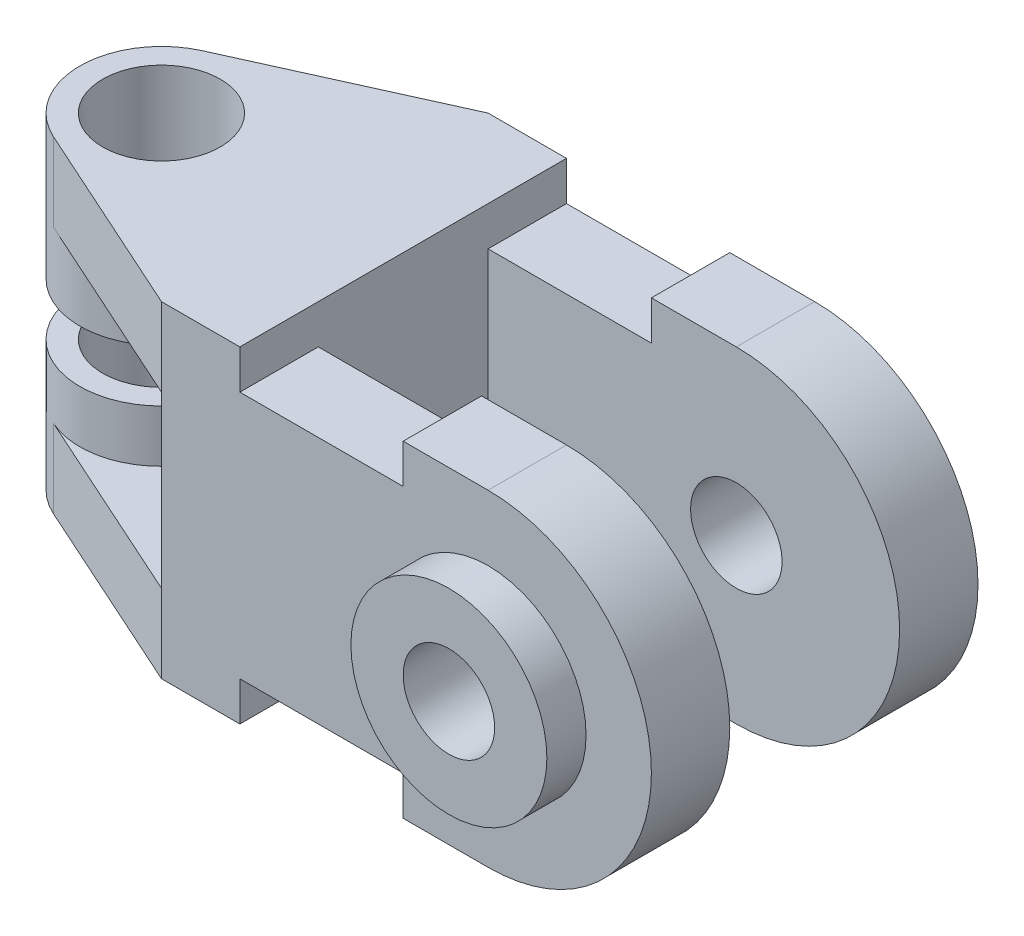
ISO-10303-21;
HEADER;
FILE_DESCRIPTION(('STEP AP214'),'2;1');
FILE_NAME('part.step','',(''),(''),'','','');
FILE_SCHEMA(('AUTOMOTIVE_DESIGN { 1 0 10303 214 1 1 1 1 }'));
ENDSEC;
DATA;
#1=APPLICATION_CONTEXT('core data for automotive mechanical design processes');
#2=APPLICATION_PROTOCOL_DEFINITION('international standard','automotive_design',2000,#1);
#3=PRODUCT_CONTEXT('',#1,'mechanical');
#4=PRODUCT('Part','Part','',(#3));
#5=PRODUCT_RELATED_PRODUCT_CATEGORY('part','',(#4));
#6=PRODUCT_DEFINITION_FORMATION('','',#4);
#7=PRODUCT_DEFINITION_CONTEXT('part definition',#1,'design');
#8=PRODUCT_DEFINITION('design','',#6,#7);
#9=PRODUCT_DEFINITION_SHAPE('','',#8);
#10=(LENGTH_UNIT() NAMED_UNIT(*) SI_UNIT(.MILLI.,.METRE.));
#11=(NAMED_UNIT(*) PLANE_ANGLE_UNIT() SI_UNIT($,.RADIAN.));
#12=(NAMED_UNIT(*) SI_UNIT($,.STERADIAN.) SOLID_ANGLE_UNIT());
#13=UNCERTAINTY_MEASURE_WITH_UNIT(LENGTH_MEASURE(1.E-05),#10,'distance_accuracy_value','');
#14=(GEOMETRIC_REPRESENTATION_CONTEXT(3) GLOBAL_UNCERTAINTY_ASSIGNED_CONTEXT((#13)) GLOBAL_UNIT_ASSIGNED_CONTEXT((#10,
#11,#12)) REPRESENTATION_CONTEXT('',''));
#15=CARTESIAN_POINT('',(0.,0.,0.));
#16=DIRECTION('',(0.,0.,1.));
#17=DIRECTION('',(1.,0.,0.));
#18=AXIS2_PLACEMENT_3D('',#15,#16,#17);
#19=CARTESIAN_POINT('',(0.,0.,12.));
#20=DIRECTION('',(1.,0.,0.));
#21=DIRECTION('',(0.,0.,-1.));
#22=AXIS2_PLACEMENT_3D('',#19,#20,#21);
#23=PLANE('',#22);
#24=DIRECTION('',(0.,0.,-1.));
#25=VECTOR('',#24,1.);
#26=CARTESIAN_POINT('',(0.,12.,0.));
#27=LINE('',#26,#25);
#28=CARTESIAN_POINT('',(0.,12.,12.));
#29=VERTEX_POINT('',#28);
#30=CARTESIAN_POINT('',(0.,12.,-38.));
#31=VERTEX_POINT('',#30);
#32=EDGE_CURVE('E62',#29,#31,#27,.T.);
#33=ORIENTED_EDGE('',*,*,#32,.F.);
#34=DIRECTION('',(0.,-1.,0.));
#35=VECTOR('',#34,1.);
#36=CARTESIAN_POINT('',(0.,0.,12.));
#37=LINE('',#36,#35);
#38=CARTESIAN_POINT('',(0.,38.,12.));
#39=VERTEX_POINT('',#38);
#40=EDGE_CURVE('E411',#39,#29,#37,.T.);
#41=ORIENTED_EDGE('',*,*,#40,.F.);
#42=DIRECTION('',(0.,0.,-1.));
#43=VECTOR('',#42,1.);
#44=CARTESIAN_POINT('',(0.,38.,-38.));
#45=LINE('',#44,#43);
#46=CARTESIAN_POINT('',(0.,38.,-38.));
#47=VERTEX_POINT('',#46);
#48=EDGE_CURVE('E265',#39,#47,#45,.T.);
#49=ORIENTED_EDGE('',*,*,#48,.T.);
#50=DIRECTION('',(0.,-1.,0.));
#51=VECTOR('',#50,1.);
#52=CARTESIAN_POINT('',(0.,50.,-38.));
#53=LINE('',#52,#51);
#54=EDGE_CURVE('E354',#47,#31,#53,.T.);
#55=ORIENTED_EDGE('',*,*,#54,.T.);
#56=EDGE_LOOP('',(#33,#41,#49,#55));
#57=FACE_BOUND('',#56,.T.);
#58=ADVANCED_FACE('F50',(#57),#23,.F.);
#59=CARTESIAN_POINT('',(12.,0.,12.));
#60=DIRECTION('',(0.,1.,0.));
#61=DIRECTION('',(0.,0.,1.));
#62=AXIS2_PLACEMENT_3D('',#59,#60,#61);
#63=PLANE('',#62);
#64=CARTESIAN_POINT('',(-24.9999999999965,0.,-13.));
#65=DIRECTION('',(0.,-1.,0.));
#66=DIRECTION('',(0.,0.,-1.));
#67=AXIS2_PLACEMENT_3D('',#64,#65,#66);
#68=CIRCLE('',#67,8.99999999999664);
#69=CARTESIAN_POINT('',(-24.9999999999965,0.,-21.9999999999966));
#70=VERTEX_POINT('',#69);
#71=EDGE_CURVE('E479',#70,#70,#68,.T.);
#72=ORIENTED_EDGE('',*,*,#71,.F.);
#73=EDGE_LOOP('',(#72));
#74=FACE_BOUND('',#73,.T.);
#75=DIRECTION('',(1.,0.,0.));
#76=VECTOR('',#75,1.);
#77=CARTESIAN_POINT('',(12.,0.,12.));
#78=LINE('',#77,#76);
#79=CARTESIAN_POINT('',(0.,0.,12.));
#80=VERTEX_POINT('',#79);
#81=CARTESIAN_POINT('',(12.,0.,12.));
#82=VERTEX_POINT('',#81);
#83=EDGE_CURVE('E249',#80,#82,#78,.T.);
#84=ORIENTED_EDGE('',*,*,#83,.F.);
#85=DIRECTION('',(-0.911437827766088,0.,-0.41143782776628));
#86=VECTOR('',#85,1.);
#87=CARTESIAN_POINT('',(-4.50000000000115,0.,9.96862696659558));
#88=LINE('',#87,#86);
#89=CARTESIAN_POINT('',(-30.1429728470736,0.,-1.60702715292695));
#90=VERTEX_POINT('',#89);
#91=EDGE_CURVE('E241',#80,#90,#88,.T.);
#92=ORIENTED_EDGE('',*,*,#91,.T.);
#93=CARTESIAN_POINT('',(-24.9999999999965,0.,-13.));
#94=DIRECTION('',(0.,-1.,0.));
#95=DIRECTION('',(0.,0.,-1.));
#96=AXIS2_PLACEMENT_3D('',#93,#94,#95);
#97=CIRCLE('',#96,12.4999999999966);
#98=CARTESIAN_POINT('',(-30.1429728470734,0.,-24.3929728470703));
#99=VERTEX_POINT('',#98);
#100=EDGE_CURVE('E224',#90,#99,#97,.T.);
#101=ORIENTED_EDGE('',*,*,#100,.T.);
#102=DIRECTION('',(-0.911437827766056,0.,0.41143782776635));
#103=VECTOR('',#102,1.);
#104=CARTESIAN_POINT('',(-14.2500000000056,0.,-31.5673187275505));
#105=LINE('',#104,#103);
#106=CARTESIAN_POINT('',(0.,0.,-38.));
#107=VERTEX_POINT('',#106);
#108=EDGE_CURVE('E255',#107,#99,#105,.T.);
#109=ORIENTED_EDGE('',*,*,#108,.F.);
#110=DIRECTION('',(-1.,0.,0.));
#111=VECTOR('',#110,1.);
#112=CARTESIAN_POINT('',(12.,0.,-38.));
#113=LINE('',#112,#111);
#114=CARTESIAN_POINT('',(12.,0.,-38.));
#115=VERTEX_POINT('',#114);
#116=EDGE_CURVE('E380',#115,#107,#113,.T.);
#117=ORIENTED_EDGE('',*,*,#116,.F.);
#118=DIRECTION('',(0.,0.,-1.));
#119=VECTOR('',#118,1.);
#120=CARTESIAN_POINT('',(12.,0.,12.));
#121=LINE('',#120,#119);
#122=EDGE_CURVE('E368',#82,#115,#121,.T.);
#123=ORIENTED_EDGE('',*,*,#122,.F.);
#124=EDGE_LOOP('',(#84,#92,#101,#109,#117,#123));
#125=FACE_BOUND('',#124,.T.);
#126=ADVANCED_FACE('F47',(#74,#125),#63,.F.);
#127=CARTESIAN_POINT('',(37.,6.,12.));
#128=DIRECTION('',(0.,1.,0.));
#129=DIRECTION('',(0.,0.,1.));
#130=AXIS2_PLACEMENT_3D('',#127,#128,#129);
#131=PLANE('',#130);
#132=DIRECTION('',(1.,0.,0.));
#133=VECTOR('',#132,1.);
#134=CARTESIAN_POINT('',(37.,6.,0.));
#135=LINE('',#134,#133);
#136=CARTESIAN_POINT('',(12.,6.,0.));
#137=VERTEX_POINT('',#136);
#138=CARTESIAN_POINT('',(37.,6.,0.));
#139=VERTEX_POINT('',#138);
#140=EDGE_CURVE('E383',#137,#139,#135,.T.);
#141=ORIENTED_EDGE('',*,*,#140,.T.);
#142=DIRECTION('',(0.,0.,-1.));
#143=VECTOR('',#142,1.);
#144=CARTESIAN_POINT('',(37.,6.,12.));
#145=LINE('',#144,#143);
#146=CARTESIAN_POINT('',(37.,6.,12.));
#147=VERTEX_POINT('',#146);
#148=EDGE_CURVE('E449',#147,#139,#145,.T.);
#149=ORIENTED_EDGE('',*,*,#148,.F.);
#150=DIRECTION('',(1.,0.,0.));
#151=VECTOR('',#150,1.);
#152=CARTESIAN_POINT('',(37.,6.,12.));
#153=LINE('',#152,#151);
#154=CARTESIAN_POINT('',(12.,6.,12.));
#155=VERTEX_POINT('',#154);
#156=EDGE_CURVE('E392',#155,#147,#153,.T.);
#157=ORIENTED_EDGE('',*,*,#156,.F.);
#158=DIRECTION('',(0.,0.,-1.));
#159=VECTOR('',#158,1.);
#160=CARTESIAN_POINT('',(12.,6.,12.));
#161=LINE('',#160,#159);
#162=EDGE_CURVE('E453',#155,#137,#161,.T.);
#163=ORIENTED_EDGE('',*,*,#162,.T.);
#164=EDGE_LOOP('',(#141,#149,#157,#163));
#165=FACE_BOUND('',#164,.T.);
#166=ADVANCED_FACE('F505',(#165),#131,.F.);
#167=CARTESIAN_POINT('',(37.,0.,12.));
#168=DIRECTION('',(1.,0.,0.));
#169=DIRECTION('',(0.,0.,-1.));
#170=AXIS2_PLACEMENT_3D('',#167,#168,#169);
#171=PLANE('',#170);
#172=DIRECTION('',(0.,-1.,0.));
#173=VECTOR('',#172,1.);
#174=CARTESIAN_POINT('',(37.,0.,0.));
#175=LINE('',#174,#173);
#176=CARTESIAN_POINT('',(37.,0.,0.));
#177=VERTEX_POINT('',#176);
#178=EDGE_CURVE('E419',#139,#177,#175,.T.);
#179=ORIENTED_EDGE('',*,*,#178,.T.);
#180=DIRECTION('',(0.,0.,-1.));
#181=VECTOR('',#180,1.);
#182=CARTESIAN_POINT('',(37.,0.,12.));
#183=LINE('',#182,#181);
#184=CARTESIAN_POINT('',(37.,0.,12.));
#185=VERTEX_POINT('',#184);
#186=EDGE_CURVE('E444',#185,#177,#183,.T.);
#187=ORIENTED_EDGE('',*,*,#186,.F.);
#188=DIRECTION('',(0.,-1.,0.));
#189=VECTOR('',#188,1.);
#190=CARTESIAN_POINT('',(37.,0.,12.));
#191=LINE('',#190,#189);
#192=EDGE_CURVE('E393',#147,#185,#191,.T.);
#193=ORIENTED_EDGE('',*,*,#192,.F.);
#194=ORIENTED_EDGE('',*,*,#148,.T.);
#195=EDGE_LOOP('',(#179,#187,#193,#194));
#196=FACE_BOUND('',#195,.T.);
#197=ADVANCED_FACE('F534',(#196),#171,.F.);
#198=CARTESIAN_POINT('',(50.,0.,12.));
#199=DIRECTION('',(0.,1.,0.));
#200=DIRECTION('',(0.,0.,1.));
#201=AXIS2_PLACEMENT_3D('',#198,#199,#200);
#202=PLANE('',#201);
#203=DIRECTION('',(1.,0.,0.));
#204=VECTOR('',#203,1.);
#205=CARTESIAN_POINT('',(50.,0.,0.));
#206=LINE('',#205,#204);
#207=CARTESIAN_POINT('',(50.,0.,0.));
#208=VERTEX_POINT('',#207);
#209=EDGE_CURVE('E416',#177,#208,#206,.T.);
#210=ORIENTED_EDGE('',*,*,#209,.T.);
#211=DIRECTION('',(0.,0.,-1.));
#212=VECTOR('',#211,1.);
#213=CARTESIAN_POINT('',(50.,0.,12.));
#214=LINE('',#213,#212);
#215=CARTESIAN_POINT('',(50.,0.,12.));
#216=VERTEX_POINT('',#215);
#217=EDGE_CURVE('E445',#216,#208,#214,.T.);
#218=ORIENTED_EDGE('',*,*,#217,.F.);
#219=DIRECTION('',(1.,0.,0.));
#220=VECTOR('',#219,1.);
#221=CARTESIAN_POINT('',(50.,0.,12.));
#222=LINE('',#221,#220);
#223=EDGE_CURVE('E397',#185,#216,#222,.T.);
#224=ORIENTED_EDGE('',*,*,#223,.F.);
#225=ORIENTED_EDGE('',*,*,#186,.T.);
#226=EDGE_LOOP('',(#210,#218,#224,#225));
#227=FACE_BOUND('',#226,.T.);
#228=ADVANCED_FACE('F528',(#227),#202,.F.);
#229=CARTESIAN_POINT('',(50.,25.,12.));
#230=DIRECTION('',(0.,0.,-1.));
#231=DIRECTION('',(-1.,0.,0.));
#232=AXIS2_PLACEMENT_3D('',#229,#230,#231);
#233=CYLINDRICAL_SURFACE('',#232,25.);
#234=CARTESIAN_POINT('',(50.,25.,0.));
#235=DIRECTION('',(0.,0.,1.));
#236=DIRECTION('',(1.,0.,0.));
#237=AXIS2_PLACEMENT_3D('',#234,#235,#236);
#238=CIRCLE('',#237,25.);
#239=CARTESIAN_POINT('',(50.,50.,0.));
#240=VERTEX_POINT('',#239);
#241=EDGE_CURVE('E423',#208,#240,#238,.T.);
#242=ORIENTED_EDGE('',*,*,#241,.T.);
#243=DIRECTION('',(0.,0.,-1.));
#244=VECTOR('',#243,1.);
#245=CARTESIAN_POINT('',(50.,50.,12.));
#246=LINE('',#245,#244);
#247=CARTESIAN_POINT('',(50.,50.,12.));
#248=VERTEX_POINT('',#247);
#249=EDGE_CURVE('E437',#248,#240,#246,.T.);
#250=ORIENTED_EDGE('',*,*,#249,.F.);
#251=CARTESIAN_POINT('',(50.,25.,12.));
#252=DIRECTION('',(0.,0.,1.));
#253=DIRECTION('',(1.,0.,0.));
#254=AXIS2_PLACEMENT_3D('',#251,#252,#253);
#255=CIRCLE('',#254,25.);
#256=EDGE_CURVE('E400',#216,#248,#255,.T.);
#257=ORIENTED_EDGE('',*,*,#256,.F.);
#258=ORIENTED_EDGE('',*,*,#217,.T.);
#259=EDGE_LOOP('',(#242,#250,#257,#258));
#260=FACE_BOUND('',#259,.T.);
#261=ADVANCED_FACE('F527',(#260),#233,.T.);
#262=CARTESIAN_POINT('',(37.,50.,12.));
#263=DIRECTION('',(0.,-1.,0.));
#264=DIRECTION('',(0.,0.,-1.));
#265=AXIS2_PLACEMENT_3D('',#262,#263,#264);
#266=PLANE('',#265);
#267=DIRECTION('',(-1.,0.,0.));
#268=VECTOR('',#267,1.);
#269=CARTESIAN_POINT('',(37.,50.,0.));
#270=LINE('',#269,#268);
#271=CARTESIAN_POINT('',(37.,50.,0.));
#272=VERTEX_POINT('',#271);
#273=EDGE_CURVE('E421',#240,#272,#270,.T.);
#274=ORIENTED_EDGE('',*,*,#273,.T.);
#275=DIRECTION('',(0.,0.,-1.));
#276=VECTOR('',#275,1.);
#277=CARTESIAN_POINT('',(37.,50.,12.));
#278=LINE('',#277,#276);
#279=CARTESIAN_POINT('',(37.,50.,12.));
#280=VERTEX_POINT('',#279);
#281=EDGE_CURVE('E436',#280,#272,#278,.T.);
#282=ORIENTED_EDGE('',*,*,#281,.F.);
#283=DIRECTION('',(-1.,0.,0.));
#284=VECTOR('',#283,1.);
#285=CARTESIAN_POINT('',(37.,50.,12.));
#286=LINE('',#285,#284);
#287=EDGE_CURVE('E398',#248,#280,#286,.T.);
#288=ORIENTED_EDGE('',*,*,#287,.F.);
#289=ORIENTED_EDGE('',*,*,#249,.T.);
#290=EDGE_LOOP('',(#274,#282,#288,#289));
#291=FACE_BOUND('',#290,.T.);
#292=ADVANCED_FACE('F522',(#291),#266,.F.);
#293=CARTESIAN_POINT('',(37.,44.,12.));
#294=DIRECTION('',(1.,0.,0.));
#295=DIRECTION('',(0.,0.,-1.));
#296=AXIS2_PLACEMENT_3D('',#293,#294,#295);
#297=PLANE('',#296);
#298=DIRECTION('',(0.,-1.,0.));
#299=VECTOR('',#298,1.);
#300=CARTESIAN_POINT('',(37.,44.,0.));
#301=LINE('',#300,#299);
#302=CARTESIAN_POINT('',(37.,44.,0.));
#303=VERTEX_POINT('',#302);
#304=EDGE_CURVE('E424',#272,#303,#301,.T.);
#305=ORIENTED_EDGE('',*,*,#304,.T.);
#306=DIRECTION('',(0.,0.,-1.));
#307=VECTOR('',#306,1.);
#308=CARTESIAN_POINT('',(37.,44.,12.));
#309=LINE('',#308,#307);
#310=CARTESIAN_POINT('',(37.,44.,12.));
#311=VERTEX_POINT('',#310);
#312=EDGE_CURVE('E433',#311,#303,#309,.T.);
#313=ORIENTED_EDGE('',*,*,#312,.F.);
#314=DIRECTION('',(0.,-1.,0.));
#315=VECTOR('',#314,1.);
#316=CARTESIAN_POINT('',(37.,44.,12.));
#317=LINE('',#316,#315);
#318=EDGE_CURVE('E405',#280,#311,#317,.T.);
#319=ORIENTED_EDGE('',*,*,#318,.F.);
#320=ORIENTED_EDGE('',*,*,#281,.T.);
#321=EDGE_LOOP('',(#305,#313,#319,#320));
#322=FACE_BOUND('',#321,.T.);
#323=ADVANCED_FACE('F517',(#322),#297,.F.);
#324=CARTESIAN_POINT('',(12.,44.,12.));
#325=DIRECTION('',(0.,-1.,0.));
#326=DIRECTION('',(0.,0.,-1.));
#327=AXIS2_PLACEMENT_3D('',#324,#325,#326);
#328=PLANE('',#327);
#329=DIRECTION('',(-1.,0.,0.));
#330=VECTOR('',#329,1.);
#331=CARTESIAN_POINT('',(12.,44.,0.));
#332=LINE('',#331,#330);
#333=CARTESIAN_POINT('',(12.,44.,0.));
#334=VERTEX_POINT('',#333);
#335=EDGE_CURVE('E386',#303,#334,#332,.T.);
#336=ORIENTED_EDGE('',*,*,#335,.T.);
#337=DIRECTION('',(0.,0.,-1.));
#338=VECTOR('',#337,1.);
#339=CARTESIAN_POINT('',(12.,44.,12.));
#340=LINE('',#339,#338);
#341=CARTESIAN_POINT('',(12.,44.,12.));
#342=VERTEX_POINT('',#341);
#343=EDGE_CURVE('E427',#342,#334,#340,.T.);
#344=ORIENTED_EDGE('',*,*,#343,.F.);
#345=DIRECTION('',(-1.,0.,0.));
#346=VECTOR('',#345,1.);
#347=CARTESIAN_POINT('',(12.,44.,12.));
#348=LINE('',#347,#346);
#349=EDGE_CURVE('E404',#311,#342,#348,.T.);
#350=ORIENTED_EDGE('',*,*,#349,.F.);
#351=ORIENTED_EDGE('',*,*,#312,.T.);
#352=EDGE_LOOP('',(#336,#344,#350,#351));
#353=FACE_BOUND('',#352,.T.);
#354=ADVANCED_FACE('F513',(#353),#328,.F.);
#355=CARTESIAN_POINT('',(12.,50.,12.));
#356=DIRECTION('',(-1.,0.,0.));
#357=DIRECTION('',(0.,0.,1.));
#358=AXIS2_PLACEMENT_3D('',#355,#356,#357);
#359=PLANE('',#358);
#360=DIRECTION('',(0.,-1.,0.));
#361=VECTOR('',#360,1.);
#362=CARTESIAN_POINT('',(12.,50.,-38.));
#363=LINE('',#362,#361);
#364=CARTESIAN_POINT('',(12.,6.00000000000001,-38.));
#365=VERTEX_POINT('',#364);
#366=EDGE_CURVE('E373',#365,#115,#363,.T.);
#367=ORIENTED_EDGE('',*,*,#366,.F.);
#368=DIRECTION('',(0.,0.,-1.));
#369=VECTOR('',#368,1.);
#370=CARTESIAN_POINT('',(12.,6.,-26.));
#371=LINE('',#370,#369);
#372=CARTESIAN_POINT('',(12.,6.,-26.));
#373=VERTEX_POINT('',#372);
#374=EDGE_CURVE('E348',#373,#365,#371,.T.);
#375=ORIENTED_EDGE('',*,*,#374,.F.);
#376=DIRECTION('',(0.,1.,0.));
#377=VECTOR('',#376,1.);
#378=CARTESIAN_POINT('',(12.,6.,-26.));
#379=LINE('',#378,#377);
#380=CARTESIAN_POINT('',(12.,44.,-26.));
#381=VERTEX_POINT('',#380);
#382=EDGE_CURVE('E304',#373,#381,#379,.T.);
#383=ORIENTED_EDGE('',*,*,#382,.T.);
#384=DIRECTION('',(0.,0.,-1.));
#385=VECTOR('',#384,1.);
#386=CARTESIAN_POINT('',(12.,44.,-26.));
#387=LINE('',#386,#385);
#388=CARTESIAN_POINT('',(12.,44.,-38.));
#389=VERTEX_POINT('',#388);
#390=EDGE_CURVE('E330',#381,#389,#387,.T.);
#391=ORIENTED_EDGE('',*,*,#390,.T.);
#392=CARTESIAN_POINT('',(12.,50.,-38.));
#393=VERTEX_POINT('',#392);
#394=EDGE_CURVE('E367',#393,#389,#363,.T.);
#395=ORIENTED_EDGE('',*,*,#394,.F.);
#396=DIRECTION('',(0.,0.,-1.));
#397=VECTOR('',#396,1.);
#398=CARTESIAN_POINT('',(12.,50.,12.));
#399=LINE('',#398,#397);
#400=CARTESIAN_POINT('',(12.,50.,12.));
#401=VERTEX_POINT('',#400);
#402=EDGE_CURVE('E415',#401,#393,#399,.T.);
#403=ORIENTED_EDGE('',*,*,#402,.F.);
#404=DIRECTION('',(0.,1.,0.));
#405=VECTOR('',#404,1.);
#406=CARTESIAN_POINT('',(12.,50.,12.));
#407=LINE('',#406,#405);
#408=EDGE_CURVE('E408',#342,#401,#407,.T.);
#409=ORIENTED_EDGE('',*,*,#408,.F.);
#410=ORIENTED_EDGE('',*,*,#343,.T.);
#411=DIRECTION('',(0.,1.,0.));
#412=VECTOR('',#411,1.);
#413=CARTESIAN_POINT('',(12.,0.,0.));
#414=LINE('',#413,#412);
#415=EDGE_CURVE('E302',#137,#334,#414,.T.);
#416=ORIENTED_EDGE('',*,*,#415,.F.);
#417=ORIENTED_EDGE('',*,*,#162,.F.);
#418=DIRECTION('',(0.,1.,0.));
#419=VECTOR('',#418,1.);
#420=CARTESIAN_POINT('',(12.,6.,12.));
#421=LINE('',#420,#419);
#422=EDGE_CURVE('E390',#82,#155,#421,.T.);
#423=ORIENTED_EDGE('',*,*,#422,.F.);
#424=ORIENTED_EDGE('',*,*,#122,.T.);
#425=EDGE_LOOP('',(#367,#375,#383,#391,#395,#403,#409,#410,#416,#417,#423,#424));
#426=FACE_BOUND('',#425,.T.);
#427=ADVANCED_FACE('F459',(#426),#359,.F.);
#428=CARTESIAN_POINT('',(0.,50.,12.));
#429=DIRECTION('',(0.,-1.,0.));
#430=DIRECTION('',(0.,0.,-1.));
#431=AXIS2_PLACEMENT_3D('',#428,#429,#430);
#432=PLANE('',#431);
#433=CARTESIAN_POINT('',(-24.9999999999965,50.,-13.));
#434=DIRECTION('',(0.,1.,0.));
#435=DIRECTION('',(0.,0.,1.));
#436=AXIS2_PLACEMENT_3D('',#433,#434,#435);
#437=CIRCLE('',#436,8.99999999999664);
#438=CARTESIAN_POINT('',(-24.9999999999965,50.,-4.00000000000335));
#439=VERTEX_POINT('',#438);
#440=EDGE_CURVE('E472',#439,#439,#437,.T.);
#441=ORIENTED_EDGE('',*,*,#440,.F.);
#442=EDGE_LOOP('',(#441));
#443=FACE_BOUND('',#442,.T.);
#444=ORIENTED_EDGE('',*,*,#402,.T.);
#445=DIRECTION('',(-1.,0.,0.));
#446=VECTOR('',#445,1.);
#447=CARTESIAN_POINT('',(12.,50.,-38.));
#448=LINE('',#447,#446);
#449=CARTESIAN_POINT('',(0.,50.,-38.));
#450=VERTEX_POINT('',#449);
#451=EDGE_CURVE('E375',#393,#450,#448,.T.);
#452=ORIENTED_EDGE('',*,*,#451,.T.);
#453=DIRECTION('',(-0.911437827766056,0.,0.41143782776635));
#454=VECTOR('',#453,1.);
#455=CARTESIAN_POINT('',(0.,50.,-38.));
#456=LINE('',#455,#454);
#457=CARTESIAN_POINT('',(-30.1429728470734,50.,-24.3929728470703));
#458=VERTEX_POINT('',#457);
#459=EDGE_CURVE('E263',#450,#458,#456,.T.);
#460=ORIENTED_EDGE('',*,*,#459,.T.);
#461=CARTESIAN_POINT('',(-24.9999999999965,50.,-13.));
#462=DIRECTION('',(0.,1.,0.));
#463=DIRECTION('',(0.,0.,1.));
#464=AXIS2_PLACEMENT_3D('',#461,#462,#463);
#465=CIRCLE('',#464,12.4999999999941);
#466=CARTESIAN_POINT('',(-30.1429728470734,50.,-1.60702715292965));
#467=VERTEX_POINT('',#466);
#468=EDGE_CURVE('E277',#458,#467,#465,.T.);
#469=ORIENTED_EDGE('',*,*,#468,.T.);
#470=DIRECTION('',(0.911437827766057,0.,0.411437827766349));
#471=VECTOR('',#470,1.);
#472=CARTESIAN_POINT('',(0.,50.,12.));
#473=LINE('',#472,#471);
#474=CARTESIAN_POINT('',(0.,50.,12.));
#475=VERTEX_POINT('',#474);
#476=EDGE_CURVE('E266',#467,#475,#473,.T.);
#477=ORIENTED_EDGE('',*,*,#476,.T.);
#478=DIRECTION('',(-1.,0.,0.));
#479=VECTOR('',#478,1.);
#480=CARTESIAN_POINT('',(0.,50.,12.));
#481=LINE('',#480,#479);
#482=EDGE_CURVE('E407',#401,#475,#481,.T.);
#483=ORIENTED_EDGE('',*,*,#482,.F.);
#484=EDGE_LOOP('',(#444,#452,#460,#469,#477,#483));
#485=FACE_BOUND('',#484,.T.);
#486=ADVANCED_FACE('F507',(#443,#485),#432,.F.);
#487=CARTESIAN_POINT('',(50.,25.,12.));
#488=DIRECTION('',(0.,0.,1.));
#489=DIRECTION('',(1.,0.,0.));
#490=AXIS2_PLACEMENT_3D('',#487,#488,#489);
#491=PLANE('',#490);
#492=CARTESIAN_POINT('',(50.,25.,12.));
#493=DIRECTION('',(0.,0.,1.));
#494=DIRECTION('',(1.,0.,0.));
#495=AXIS2_PLACEMENT_3D('',#492,#493,#494);
#496=CIRCLE('',#495,15.);
#497=CARTESIAN_POINT('',(65.,25.,12.));
#498=VERTEX_POINT('',#497);
#499=EDGE_CURVE('E378',#498,#498,#496,.T.);
#500=ORIENTED_EDGE('',*,*,#499,.F.);
#501=EDGE_LOOP('',(#500));
#502=FACE_BOUND('',#501,.T.);
#503=ORIENTED_EDGE('',*,*,#83,.T.);
#504=ORIENTED_EDGE('',*,*,#422,.T.);
#505=ORIENTED_EDGE('',*,*,#156,.T.);
#506=ORIENTED_EDGE('',*,*,#192,.T.);
#507=ORIENTED_EDGE('',*,*,#223,.T.);
#508=ORIENTED_EDGE('',*,*,#256,.T.);
#509=ORIENTED_EDGE('',*,*,#287,.T.);
#510=ORIENTED_EDGE('',*,*,#318,.T.);
#511=ORIENTED_EDGE('',*,*,#349,.T.);
#512=ORIENTED_EDGE('',*,*,#408,.T.);
#513=ORIENTED_EDGE('',*,*,#482,.T.);
#514=EDGE_CURVE('E412',#475,#39,#37,.T.);
#515=ORIENTED_EDGE('',*,*,#514,.T.);
#516=ORIENTED_EDGE('',*,*,#40,.T.);
#517=DIRECTION('',(0.,-1.,0.));
#518=VECTOR('',#517,1.);
#519=CARTESIAN_POINT('',(0.,12.,12.));
#520=LINE('',#519,#518);
#521=EDGE_CURVE('E244',#29,#80,#520,.T.);
#522=ORIENTED_EDGE('',*,*,#521,.T.);
#523=EDGE_LOOP('',(#503,#504,#505,#506,#507,#508,#509,#510,#511,#512,#513,#515,#516,#522));
#524=FACE_BOUND('',#523,.T.);
#525=ADVANCED_FACE('F512',(#502,#524),#491,.T.);
#526=CARTESIAN_POINT('',(50.,25.,0.));
#527=DIRECTION('',(0.,0.,1.));
#528=DIRECTION('',(1.,0.,0.));
#529=AXIS2_PLACEMENT_3D('',#526,#527,#528);
#530=PLANE('',#529);
#531=CARTESIAN_POINT('',(50.,25.,0.));
#532=DIRECTION('',(0.,0.,1.));
#533=DIRECTION('',(1.,0.,0.));
#534=AXIS2_PLACEMENT_3D('',#531,#532,#533);
#535=CIRCLE('',#534,7.);
#536=CARTESIAN_POINT('',(57.,25.,0.));
#537=VERTEX_POINT('',#536);
#538=EDGE_CURVE('E289',#537,#537,#535,.T.);
#539=ORIENTED_EDGE('',*,*,#538,.T.);
#540=EDGE_LOOP('',(#539));
#541=FACE_BOUND('',#540,.T.);
#542=ORIENTED_EDGE('',*,*,#140,.F.);
#543=ORIENTED_EDGE('',*,*,#415,.T.);
#544=ORIENTED_EDGE('',*,*,#335,.F.);
#545=ORIENTED_EDGE('',*,*,#304,.F.);
#546=ORIENTED_EDGE('',*,*,#273,.F.);
#547=ORIENTED_EDGE('',*,*,#241,.F.);
#548=ORIENTED_EDGE('',*,*,#209,.F.);
#549=ORIENTED_EDGE('',*,*,#178,.F.);
#550=EDGE_LOOP('',(#542,#543,#544,#545,#546,#547,#548,#549));
#551=FACE_BOUND('',#550,.T.);
#552=ADVANCED_FACE('F506',(#541,#551),#530,.F.);
#553=CARTESIAN_POINT('',(50.,25.,18.));
#554=DIRECTION('',(0.,0.,-1.));
#555=DIRECTION('',(-1.,0.,0.));
#556=AXIS2_PLACEMENT_3D('',#553,#554,#555);
#557=CYLINDRICAL_SURFACE('',#556,15.);
#558=CARTESIAN_POINT('',(50.,25.,18.));
#559=DIRECTION('',(0.,0.,1.));
#560=DIRECTION('',(1.,0.,0.));
#561=AXIS2_PLACEMENT_3D('',#558,#559,#560);
#562=CIRCLE('',#561,15.);
#563=CARTESIAN_POINT('',(65.,25.,18.));
#564=VERTEX_POINT('',#563);
#565=EDGE_CURVE('E385',#564,#564,#562,.T.);
#566=ORIENTED_EDGE('',*,*,#565,.F.);
#567=EDGE_LOOP('',(#566));
#568=FACE_BOUND('',#567,.T.);
#569=ORIENTED_EDGE('',*,*,#499,.T.);
#570=EDGE_LOOP('',(#569));
#571=FACE_BOUND('',#570,.T.);
#572=ADVANCED_FACE('F665',(#568,#571),#557,.T.);
#573=CARTESIAN_POINT('',(50.,25.,18.));
#574=DIRECTION('',(0.,0.,1.));
#575=DIRECTION('',(1.,0.,0.));
#576=AXIS2_PLACEMENT_3D('',#573,#574,#575);
#577=PLANE('',#576);
#578=CARTESIAN_POINT('',(50.,25.,18.));
#579=DIRECTION('',(0.,0.,1.));
#580=DIRECTION('',(1.,0.,0.));
#581=AXIS2_PLACEMENT_3D('',#578,#579,#580);
#582=CIRCLE('',#581,7.);
#583=CARTESIAN_POINT('',(57.,25.,18.));
#584=VERTEX_POINT('',#583);
#585=EDGE_CURVE('E285',#584,#584,#582,.T.);
#586=ORIENTED_EDGE('',*,*,#585,.F.);
#587=EDGE_LOOP('',(#586));
#588=FACE_BOUND('',#587,.T.);
#589=ORIENTED_EDGE('',*,*,#565,.T.);
#590=EDGE_LOOP('',(#589));
#591=FACE_BOUND('',#590,.T.);
#592=ADVANCED_FACE('F660',(#588,#591),#577,.T.);
#593=CARTESIAN_POINT('',(12.,50.,-38.));
#594=DIRECTION('',(0.,0.,-1.));
#595=DIRECTION('',(-1.,0.,0.));
#596=AXIS2_PLACEMENT_3D('',#593,#594,#595);
#597=PLANE('',#596);
#598=CARTESIAN_POINT('',(49.9999999999999,25.,-38.));
#599=DIRECTION('',(0.,0.,-1.));
#600=DIRECTION('',(-1.,0.,0.));
#601=AXIS2_PLACEMENT_3D('',#598,#599,#600);
#602=CIRCLE('',#601,15.);
#603=CARTESIAN_POINT('',(34.9999999999999,25.,-38.));
#604=VERTEX_POINT('',#603);
#605=EDGE_CURVE('E57',#604,#604,#602,.T.);
#606=ORIENTED_EDGE('',*,*,#605,.F.);
#607=EDGE_LOOP('',(#606));
#608=FACE_BOUND('',#607,.T.);
#609=EDGE_CURVE('E372',#450,#47,#53,.T.);
#610=ORIENTED_EDGE('',*,*,#609,.F.);
#611=ORIENTED_EDGE('',*,*,#451,.F.);
#612=ORIENTED_EDGE('',*,*,#394,.T.);
#613=DIRECTION('',(1.,0.,0.));
#614=VECTOR('',#613,1.);
#615=CARTESIAN_POINT('',(12.,44.,-38.));
#616=LINE('',#615,#614);
#617=CARTESIAN_POINT('',(37.,44.,-38.));
#618=VERTEX_POINT('',#617);
#619=EDGE_CURVE('E301',#389,#618,#616,.T.);
#620=ORIENTED_EDGE('',*,*,#619,.T.);
#621=DIRECTION('',(0.,1.,0.));
#622=VECTOR('',#621,1.);
#623=CARTESIAN_POINT('',(37.,44.,-38.));
#624=LINE('',#623,#622);
#625=CARTESIAN_POINT('',(37.,50.,-38.));
#626=VERTEX_POINT('',#625);
#627=EDGE_CURVE('E335',#618,#626,#624,.T.);
#628=ORIENTED_EDGE('',*,*,#627,.T.);
#629=DIRECTION('',(1.,0.,0.));
#630=VECTOR('',#629,1.);
#631=CARTESIAN_POINT('',(37.,50.,-38.));
#632=LINE('',#631,#630);
#633=CARTESIAN_POINT('',(50.,50.,-38.));
#634=VERTEX_POINT('',#633);
#635=EDGE_CURVE('E337',#626,#634,#632,.T.);
#636=ORIENTED_EDGE('',*,*,#635,.T.);
#637=CARTESIAN_POINT('',(49.9999999999999,25.,-38.));
#638=DIRECTION('',(0.,0.,-1.));
#639=DIRECTION('',(-1.,0.,0.));
#640=AXIS2_PLACEMENT_3D('',#637,#638,#639);
#641=CIRCLE('',#640,25.);
#642=CARTESIAN_POINT('',(49.9999999999998,0.,-38.));
#643=VERTEX_POINT('',#642);
#644=EDGE_CURVE('E339',#634,#643,#641,.T.);
#645=ORIENTED_EDGE('',*,*,#644,.T.);
#646=DIRECTION('',(-1.,0.,0.));
#647=VECTOR('',#646,1.);
#648=CARTESIAN_POINT('',(49.9999999999998,0.,-38.));
#649=LINE('',#648,#647);
#650=CARTESIAN_POINT('',(37.,0.,-38.));
#651=VERTEX_POINT('',#650);
#652=EDGE_CURVE('E344',#643,#651,#649,.T.);
#653=ORIENTED_EDGE('',*,*,#652,.T.);
#654=DIRECTION('',(0.,1.,0.));
#655=VECTOR('',#654,1.);
#656=CARTESIAN_POINT('',(37.,0.,-38.));
#657=LINE('',#656,#655);
#658=CARTESIAN_POINT('',(37.,6.,-38.));
#659=VERTEX_POINT('',#658);
#660=EDGE_CURVE('E341',#651,#659,#657,.T.);
#661=ORIENTED_EDGE('',*,*,#660,.T.);
#662=DIRECTION('',(-1.,0.,0.));
#663=VECTOR('',#662,1.);
#664=CARTESIAN_POINT('',(37.,6.,-38.));
#665=LINE('',#664,#663);
#666=EDGE_CURVE('E307',#659,#365,#665,.T.);
#667=ORIENTED_EDGE('',*,*,#666,.T.);
#668=ORIENTED_EDGE('',*,*,#366,.T.);
#669=ORIENTED_EDGE('',*,*,#116,.T.);
#670=DIRECTION('',(0.,-1.,0.));
#671=VECTOR('',#670,1.);
#672=CARTESIAN_POINT('',(0.,12.,-38.));
#673=LINE('',#672,#671);
#674=EDGE_CURVE('E72',#31,#107,#673,.T.);
#675=ORIENTED_EDGE('',*,*,#674,.F.);
#676=ORIENTED_EDGE('',*,*,#54,.F.);
#677=EDGE_LOOP('',(#610,#611,#612,#620,#628,#636,#645,#653,#661,#667,#668,#669,#675,#676));
#678=FACE_BOUND('',#677,.T.);
#679=ADVANCED_FACE('F464',(#608,#678),#597,.T.);
#680=CARTESIAN_POINT('',(37.,6.,-26.));
#681=DIRECTION('',(0.,-1.,0.));
#682=DIRECTION('',(0.,0.,-1.));
#683=AXIS2_PLACEMENT_3D('',#680,#681,#682);
#684=PLANE('',#683);
#685=ORIENTED_EDGE('',*,*,#666,.F.);
#686=DIRECTION('',(0.,0.,-1.));
#687=VECTOR('',#686,1.);
#688=CARTESIAN_POINT('',(37.,6.,-26.));
#689=LINE('',#688,#687);
#690=CARTESIAN_POINT('',(37.,6.,-26.));
#691=VERTEX_POINT('',#690);
#692=EDGE_CURVE('E355',#691,#659,#689,.T.);
#693=ORIENTED_EDGE('',*,*,#692,.F.);
#694=DIRECTION('',(-1.,0.,0.));
#695=VECTOR('',#694,1.);
#696=CARTESIAN_POINT('',(37.,6.,-26.));
#697=LINE('',#696,#695);
#698=EDGE_CURVE('E327',#691,#373,#697,.T.);
#699=ORIENTED_EDGE('',*,*,#698,.T.);
#700=ORIENTED_EDGE('',*,*,#374,.T.);
#701=EDGE_LOOP('',(#685,#693,#699,#700));
#702=FACE_BOUND('',#701,.T.);
#703=ADVANCED_FACE('F627',(#702),#684,.T.);
#704=CARTESIAN_POINT('',(37.,0.,-26.));
#705=DIRECTION('',(-1.,0.,0.));
#706=DIRECTION('',(0.,0.,1.));
#707=AXIS2_PLACEMENT_3D('',#704,#705,#706);
#708=PLANE('',#707);
#709=ORIENTED_EDGE('',*,*,#660,.F.);
#710=DIRECTION('',(0.,0.,-1.));
#711=VECTOR('',#710,1.);
#712=CARTESIAN_POINT('',(37.,0.,-26.));
#713=LINE('',#712,#711);
#714=CARTESIAN_POINT('',(37.,0.,-26.));
#715=VERTEX_POINT('',#714);
#716=EDGE_CURVE('E353',#715,#651,#713,.T.);
#717=ORIENTED_EDGE('',*,*,#716,.F.);
#718=DIRECTION('',(0.,1.,0.));
#719=VECTOR('',#718,1.);
#720=CARTESIAN_POINT('',(37.,0.,-26.));
#721=LINE('',#720,#719);
#722=EDGE_CURVE('E325',#715,#691,#721,.T.);
#723=ORIENTED_EDGE('',*,*,#722,.T.);
#724=ORIENTED_EDGE('',*,*,#692,.T.);
#725=EDGE_LOOP('',(#709,#717,#723,#724));
#726=FACE_BOUND('',#725,.T.);
#727=ADVANCED_FACE('F635',(#726),#708,.T.);
#728=CARTESIAN_POINT('',(49.9999999999998,0.,-26.));
#729=DIRECTION('',(0.,-1.,0.));
#730=DIRECTION('',(0.,0.,-1.));
#731=AXIS2_PLACEMENT_3D('',#728,#729,#730);
#732=PLANE('',#731);
#733=ORIENTED_EDGE('',*,*,#652,.F.);
#734=DIRECTION('',(0.,0.,-1.));
#735=VECTOR('',#734,1.);
#736=CARTESIAN_POINT('',(49.9999999999998,0.,-26.));
#737=LINE('',#736,#735);
#738=CARTESIAN_POINT('',(49.9999999999998,0.,-26.));
#739=VERTEX_POINT('',#738);
#740=EDGE_CURVE('E357',#739,#643,#737,.T.);
#741=ORIENTED_EDGE('',*,*,#740,.F.);
#742=DIRECTION('',(-1.,0.,0.));
#743=VECTOR('',#742,1.);
#744=CARTESIAN_POINT('',(49.9999999999998,0.,-26.));
#745=LINE('',#744,#743);
#746=EDGE_CURVE('E323',#739,#715,#745,.T.);
#747=ORIENTED_EDGE('',*,*,#746,.T.);
#748=ORIENTED_EDGE('',*,*,#716,.T.);
#749=EDGE_LOOP('',(#733,#741,#747,#748));
#750=FACE_BOUND('',#749,.T.);
#751=ADVANCED_FACE('F636',(#750),#732,.T.);
#752=CARTESIAN_POINT('',(49.9999999999999,25.,-26.));
#753=DIRECTION('',(0.,0.,-1.));
#754=DIRECTION('',(-1.,0.,0.));
#755=AXIS2_PLACEMENT_3D('',#752,#753,#754);
#756=CYLINDRICAL_SURFACE('',#755,25.);
#757=ORIENTED_EDGE('',*,*,#644,.F.);
#758=DIRECTION('',(0.,0.,-1.));
#759=VECTOR('',#758,1.);
#760=CARTESIAN_POINT('',(50.,50.,-26.));
#761=LINE('',#760,#759);
#762=CARTESIAN_POINT('',(50.,50.,-26.));
#763=VERTEX_POINT('',#762);
#764=EDGE_CURVE('E360',#763,#634,#761,.T.);
#765=ORIENTED_EDGE('',*,*,#764,.F.);
#766=CARTESIAN_POINT('',(49.9999999999999,25.,-26.));
#767=DIRECTION('',(0.,0.,-1.));
#768=DIRECTION('',(-1.,0.,0.));
#769=AXIS2_PLACEMENT_3D('',#766,#767,#768);
#770=CIRCLE('',#769,25.);
#771=EDGE_CURVE('E319',#763,#739,#770,.T.);
#772=ORIENTED_EDGE('',*,*,#771,.T.);
#773=ORIENTED_EDGE('',*,*,#740,.T.);
#774=EDGE_LOOP('',(#757,#765,#772,#773));
#775=FACE_BOUND('',#774,.T.);
#776=ADVANCED_FACE('F639',(#775),#756,.T.);
#777=CARTESIAN_POINT('',(37.,50.,-26.));
#778=DIRECTION('',(0.,1.,0.));
#779=DIRECTION('',(0.,0.,1.));
#780=AXIS2_PLACEMENT_3D('',#777,#778,#779);
#781=PLANE('',#780);
#782=ORIENTED_EDGE('',*,*,#635,.F.);
#783=DIRECTION('',(0.,0.,-1.));
#784=VECTOR('',#783,1.);
#785=CARTESIAN_POINT('',(37.,50.,-26.));
#786=LINE('',#785,#784);
#787=CARTESIAN_POINT('',(37.,50.,-26.));
#788=VERTEX_POINT('',#787);
#789=EDGE_CURVE('E363',#788,#626,#786,.T.);
#790=ORIENTED_EDGE('',*,*,#789,.F.);
#791=DIRECTION('',(1.,0.,0.));
#792=VECTOR('',#791,1.);
#793=CARTESIAN_POINT('',(37.,50.,-26.));
#794=LINE('',#793,#792);
#795=EDGE_CURVE('E314',#788,#763,#794,.T.);
#796=ORIENTED_EDGE('',*,*,#795,.T.);
#797=ORIENTED_EDGE('',*,*,#764,.T.);
#798=EDGE_LOOP('',(#782,#790,#796,#797));
#799=FACE_BOUND('',#798,.T.);
#800=ADVANCED_FACE('F641',(#799),#781,.T.);
#801=CARTESIAN_POINT('',(37.,44.,-26.));
#802=DIRECTION('',(-1.,0.,0.));
#803=DIRECTION('',(0.,0.,1.));
#804=AXIS2_PLACEMENT_3D('',#801,#802,#803);
#805=PLANE('',#804);
#806=ORIENTED_EDGE('',*,*,#627,.F.);
#807=DIRECTION('',(0.,0.,-1.));
#808=VECTOR('',#807,1.);
#809=CARTESIAN_POINT('',(37.,44.,-26.));
#810=LINE('',#809,#808);
#811=CARTESIAN_POINT('',(37.,44.,-26.));
#812=VERTEX_POINT('',#811);
#813=EDGE_CURVE('E361',#812,#618,#810,.T.);
#814=ORIENTED_EDGE('',*,*,#813,.F.);
#815=DIRECTION('',(0.,1.,0.));
#816=VECTOR('',#815,1.);
#817=CARTESIAN_POINT('',(37.,44.,-26.));
#818=LINE('',#817,#816);
#819=EDGE_CURVE('E315',#812,#788,#818,.T.);
#820=ORIENTED_EDGE('',*,*,#819,.T.);
#821=ORIENTED_EDGE('',*,*,#789,.T.);
#822=EDGE_LOOP('',(#806,#814,#820,#821));
#823=FACE_BOUND('',#822,.T.);
#824=ADVANCED_FACE('F647',(#823),#805,.T.);
#825=CARTESIAN_POINT('',(12.,44.,-26.));
#826=DIRECTION('',(0.,1.,0.));
#827=DIRECTION('',(0.,0.,1.));
#828=AXIS2_PLACEMENT_3D('',#825,#826,#827);
#829=PLANE('',#828);
#830=ORIENTED_EDGE('',*,*,#619,.F.);
#831=ORIENTED_EDGE('',*,*,#390,.F.);
#832=DIRECTION('',(1.,0.,0.));
#833=VECTOR('',#832,1.);
#834=CARTESIAN_POINT('',(12.,44.,-26.));
#835=LINE('',#834,#833);
#836=EDGE_CURVE('E308',#381,#812,#835,.T.);
#837=ORIENTED_EDGE('',*,*,#836,.T.);
#838=ORIENTED_EDGE('',*,*,#813,.T.);
#839=EDGE_LOOP('',(#830,#831,#837,#838));
#840=FACE_BOUND('',#839,.T.);
#841=ADVANCED_FACE('F630',(#840),#829,.T.);
#842=CARTESIAN_POINT('',(49.9999999999999,25.,-26.));
#843=DIRECTION('',(0.,0.,-1.));
#844=DIRECTION('',(-1.,0.,0.));
#845=AXIS2_PLACEMENT_3D('',#842,#843,#844);
#846=PLANE('',#845);
#847=CARTESIAN_POINT('',(49.9999999999999,25.,-26.));
#848=DIRECTION('',(0.,0.,-1.));
#849=DIRECTION('',(-1.,0.,0.));
#850=AXIS2_PLACEMENT_3D('',#847,#848,#849);
#851=CIRCLE('',#850,7.);
#852=CARTESIAN_POINT('',(42.9999999999999,25.,-26.));
#853=VERTEX_POINT('',#852);
#854=EDGE_CURVE('E291',#853,#853,#851,.T.);
#855=ORIENTED_EDGE('',*,*,#854,.T.);
#856=EDGE_LOOP('',(#855));
#857=FACE_BOUND('',#856,.T.);
#858=ORIENTED_EDGE('',*,*,#382,.F.);
#859=ORIENTED_EDGE('',*,*,#698,.F.);
#860=ORIENTED_EDGE('',*,*,#722,.F.);
#861=ORIENTED_EDGE('',*,*,#746,.F.);
#862=ORIENTED_EDGE('',*,*,#771,.F.);
#863=ORIENTED_EDGE('',*,*,#795,.F.);
#864=ORIENTED_EDGE('',*,*,#819,.F.);
#865=ORIENTED_EDGE('',*,*,#836,.F.);
#866=EDGE_LOOP('',(#858,#859,#860,#861,#862,#863,#864,#865));
#867=FACE_BOUND('',#866,.T.);
#868=ADVANCED_FACE('F621',(#857,#867),#846,.F.);
#869=CARTESIAN_POINT('',(49.9999999999999,25.,-44.));
#870=DIRECTION('',(0.,0.,1.));
#871=DIRECTION('',(1.,0.,0.));
#872=AXIS2_PLACEMENT_3D('',#869,#870,#871);
#873=CYLINDRICAL_SURFACE('',#872,15.);
#874=CARTESIAN_POINT('',(49.9999999999999,25.,-44.));
#875=DIRECTION('',(0.,0.,-1.));
#876=DIRECTION('',(-1.,0.,0.));
#877=AXIS2_PLACEMENT_3D('',#874,#875,#876);
#878=CIRCLE('',#877,15.);
#879=CARTESIAN_POINT('',(34.9999999999999,25.,-44.));
#880=VERTEX_POINT('',#879);
#881=EDGE_CURVE('E298',#880,#880,#878,.T.);
#882=ORIENTED_EDGE('',*,*,#881,.F.);
#883=EDGE_LOOP('',(#882));
#884=FACE_BOUND('',#883,.T.);
#885=ORIENTED_EDGE('',*,*,#605,.T.);
#886=EDGE_LOOP('',(#885));
#887=FACE_BOUND('',#886,.T.);
#888=ADVANCED_FACE('F620',(#884,#887),#873,.T.);
#889=CARTESIAN_POINT('',(49.9999999999999,25.,-44.));
#890=DIRECTION('',(0.,0.,-1.));
#891=DIRECTION('',(-1.,0.,0.));
#892=AXIS2_PLACEMENT_3D('',#889,#890,#891);
#893=PLANE('',#892);
#894=CARTESIAN_POINT('',(49.9999999999999,25.,-44.));
#895=DIRECTION('',(0.,0.,-1.));
#896=DIRECTION('',(-1.,0.,0.));
#897=AXIS2_PLACEMENT_3D('',#894,#895,#896);
#898=CIRCLE('',#897,7.);
#899=CARTESIAN_POINT('',(42.9999999999999,25.,-44.));
#900=VERTEX_POINT('',#899);
#901=EDGE_CURVE('E288',#900,#900,#898,.T.);
#902=ORIENTED_EDGE('',*,*,#901,.F.);
#903=EDGE_LOOP('',(#902));
#904=FACE_BOUND('',#903,.T.);
#905=ORIENTED_EDGE('',*,*,#881,.T.);
#906=EDGE_LOOP('',(#905));
#907=FACE_BOUND('',#906,.T.);
#908=ADVANCED_FACE('F613',(#904,#907),#893,.T.);
#909=CARTESIAN_POINT('',(49.9999999999999,25.,-26.));
#910=DIRECTION('',(0.,0.,-1.));
#911=DIRECTION('',(-1.,0.,0.));
#912=AXIS2_PLACEMENT_3D('',#909,#910,#911);
#913=CYLINDRICAL_SURFACE('',#912,7.);
#914=ORIENTED_EDGE('',*,*,#854,.F.);
#915=EDGE_LOOP('',(#914));
#916=FACE_BOUND('',#915,.T.);
#917=ORIENTED_EDGE('',*,*,#901,.T.);
#918=EDGE_LOOP('',(#917));
#919=FACE_BOUND('',#918,.T.);
#920=ADVANCED_FACE('F612',(#916,#919),#913,.F.);
#921=CARTESIAN_POINT('',(50.,25.,0.));
#922=DIRECTION('',(0.,0.,1.));
#923=DIRECTION('',(1.,0.,0.));
#924=AXIS2_PLACEMENT_3D('',#921,#922,#923);
#925=CYLINDRICAL_SURFACE('',#924,7.);
#926=ORIENTED_EDGE('',*,*,#538,.F.);
#927=EDGE_LOOP('',(#926));
#928=FACE_BOUND('',#927,.T.);
#929=ORIENTED_EDGE('',*,*,#585,.T.);
#930=EDGE_LOOP('',(#929));
#931=FACE_BOUND('',#930,.T.);
#932=ADVANCED_FACE('F604',(#928,#931),#925,.F.);
#933=CARTESIAN_POINT('',(0.,38.,12.));
#934=DIRECTION('',(-0.411437827766349,0.,0.911437827766057));
#935=DIRECTION('',(0.911437827766057,0.,0.411437827766349));
#936=AXIS2_PLACEMENT_3D('',#933,#934,#935);
#937=PLANE('',#936);
#938=ORIENTED_EDGE('',*,*,#476,.F.);
#939=DIRECTION('',(0.,1.,0.));
#940=VECTOR('',#939,1.);
#941=CARTESIAN_POINT('',(-30.1429728470734,38.,-1.60702715292965));
#942=LINE('',#941,#940);
#943=CARTESIAN_POINT('',(-30.1429728470745,38.,-1.60702715292735));
#944=VERTEX_POINT('',#943);
#945=EDGE_CURVE('E284',#944,#467,#942,.T.);
#946=ORIENTED_EDGE('',*,*,#945,.F.);
#947=DIRECTION('',(0.911437827766057,0.,0.411437827766349));
#948=VECTOR('',#947,1.);
#949=CARTESIAN_POINT('',(0.,38.,12.));
#950=LINE('',#949,#948);
#951=EDGE_CURVE('E275',#944,#39,#950,.T.);
#952=ORIENTED_EDGE('',*,*,#951,.T.);
#953=ORIENTED_EDGE('',*,*,#514,.F.);
#954=EDGE_LOOP('',(#938,#946,#952,#953));
#955=FACE_BOUND('',#954,.T.);
#956=ADVANCED_FACE('F574',(#955),#937,.T.);
#957=CARTESIAN_POINT('',(-24.9999999999965,38.,-13.));
#958=DIRECTION('',(0.,1.,0.));
#959=DIRECTION('',(0.,0.,1.));
#960=AXIS2_PLACEMENT_3D('',#957,#958,#959);
#961=CYLINDRICAL_SURFACE('',#960,12.4999999999941);
#962=ORIENTED_EDGE('',*,*,#468,.F.);
#963=DIRECTION('',(0.,1.,0.));
#964=VECTOR('',#963,1.);
#965=CARTESIAN_POINT('',(-30.1429728470734,38.,-24.3929728470703));
#966=LINE('',#965,#964);
#967=CARTESIAN_POINT('',(-30.1429728470734,38.,-24.3929728470703));
#968=VERTEX_POINT('',#967);
#969=EDGE_CURVE('E273',#968,#458,#966,.T.);
#970=ORIENTED_EDGE('',*,*,#969,.F.);
#971=CARTESIAN_POINT('',(-24.9999999999965,38.,-13.));
#972=DIRECTION('',(0.,1.,0.));
#973=DIRECTION('',(0.,0.,1.));
#974=AXIS2_PLACEMENT_3D('',#971,#972,#973);
#975=CIRCLE('',#974,12.4999999999966);
#976=EDGE_CURVE('E11',#968,#944,#975,.F.);
#977=ORIENTED_EDGE('',*,*,#976,.T.);
#978=ORIENTED_EDGE('',*,*,#945,.T.);
#979=EDGE_LOOP('',(#962,#970,#977,#978));
#980=FACE_BOUND('',#979,.T.);
#981=CARTESIAN_POINT('',(-24.9999999999965,28.,-13.));
#982=DIRECTION('',(0.,-1.,0.));
#983=DIRECTION('',(0.,0.,-1.));
#984=AXIS2_PLACEMENT_3D('',#981,#982,#983);
#985=CIRCLE('',#984,12.4999999999966);
#986=CARTESIAN_POINT('',(-24.9999999999965,28.,-25.4999999999966));
#987=VERTEX_POINT('',#986);
#988=EDGE_CURVE('E242',#987,#987,#985,.T.);
#989=ORIENTED_EDGE('',*,*,#988,.F.);
#990=EDGE_LOOP('',(#989));
#991=FACE_BOUND('',#990,.T.);
#992=ADVANCED_FACE('F603',(#980,#991),#961,.T.);
#993=CARTESIAN_POINT('',(0.,38.,-38.));
#994=DIRECTION('',(-0.41143782776635,0.,-0.911437827766056));
#995=DIRECTION('',(-0.911437827766056,0.,0.41143782776635));
#996=AXIS2_PLACEMENT_3D('',#993,#994,#995);
#997=PLANE('',#996);
#998=ORIENTED_EDGE('',*,*,#459,.F.);
#999=ORIENTED_EDGE('',*,*,#609,.T.);
#1000=DIRECTION('',(-0.911437827766056,0.,0.41143782776635));
#1001=VECTOR('',#1000,1.);
#1002=CARTESIAN_POINT('',(0.,38.,-38.));
#1003=LINE('',#1002,#1001);
#1004=EDGE_CURVE('E270',#47,#968,#1003,.T.);
#1005=ORIENTED_EDGE('',*,*,#1004,.T.);
#1006=ORIENTED_EDGE('',*,*,#969,.T.);
#1007=EDGE_LOOP('',(#998,#999,#1005,#1006));
#1008=FACE_BOUND('',#1007,.T.);
#1009=ADVANCED_FACE('F600',(#1008),#997,.T.);
#1010=CARTESIAN_POINT('',(-24.9999999999965,38.,-13.));
#1011=DIRECTION('',(0.,1.,0.));
#1012=DIRECTION('',(0.,0.,1.));
#1013=AXIS2_PLACEMENT_3D('',#1010,#1011,#1012);
#1014=PLANE('',#1013);
#1015=ORIENTED_EDGE('',*,*,#976,.F.);
#1016=ORIENTED_EDGE('',*,*,#1004,.F.);
#1017=ORIENTED_EDGE('',*,*,#48,.F.);
#1018=ORIENTED_EDGE('',*,*,#951,.F.);
#1019=EDGE_LOOP('',(#1015,#1016,#1017,#1018));
#1020=FACE_BOUND('',#1019,.T.);
#1021=ADVANCED_FACE('F595',(#1020),#1014,.F.);
#1022=CARTESIAN_POINT('',(-24.9999999999965,28.,-13.));
#1023=DIRECTION('',(0.,-1.,0.));
#1024=DIRECTION('',(0.,0.,-1.));
#1025=AXIS2_PLACEMENT_3D('',#1022,#1023,#1024);
#1026=PLANE('',#1025);
#1027=CARTESIAN_POINT('',(-24.9999999999965,28.,-13.));
#1028=DIRECTION('',(0.,1.,0.));
#1029=DIRECTION('',(0.,0.,1.));
#1030=AXIS2_PLACEMENT_3D('',#1027,#1028,#1029);
#1031=CIRCLE('',#1030,8.99999999999664);
#1032=CARTESIAN_POINT('',(-24.9999999999965,28.,-4.00000000000335));
#1033=VERTEX_POINT('',#1032);
#1034=EDGE_CURVE('E234',#1033,#1033,#1031,.T.);
#1035=ORIENTED_EDGE('',*,*,#1034,.T.);
#1036=EDGE_LOOP('',(#1035));
#1037=FACE_BOUND('',#1036,.T.);
#1038=ORIENTED_EDGE('',*,*,#988,.T.);
#1039=EDGE_LOOP('',(#1038));
#1040=FACE_BOUND('',#1039,.T.);
#1041=ADVANCED_FACE('F588',(#1037,#1040),#1026,.T.);
#1042=CARTESIAN_POINT('',(-4.50000000000115,12.,9.96862696659558));
#1043=DIRECTION('',(-0.41143782776628,0.,0.911437827766088));
#1044=DIRECTION('',(0.911437827766088,0.,0.41143782776628));
#1045=AXIS2_PLACEMENT_3D('',#1042,#1043,#1044);
#1046=PLANE('',#1045);
#1047=ORIENTED_EDGE('',*,*,#91,.F.);
#1048=ORIENTED_EDGE('',*,*,#521,.F.);
#1049=DIRECTION('',(-0.911437827766088,0.,-0.41143782776628));
#1050=VECTOR('',#1049,1.);
#1051=CARTESIAN_POINT('',(-4.50000000000115,12.,9.96862696659558));
#1052=LINE('',#1051,#1050);
#1053=CARTESIAN_POINT('',(-30.1429728470745,12.,-1.60702715292735));
#1054=VERTEX_POINT('',#1053);
#1055=EDGE_CURVE('E243',#29,#1054,#1052,.T.);
#1056=ORIENTED_EDGE('',*,*,#1055,.T.);
#1057=DIRECTION('',(0.,-1.,0.));
#1058=VECTOR('',#1057,1.);
#1059=CARTESIAN_POINT('',(-30.1429728470745,12.,-1.60702715292735));
#1060=LINE('',#1059,#1058);
#1061=EDGE_CURVE('E223',#1054,#90,#1060,.T.);
#1062=ORIENTED_EDGE('',*,*,#1061,.T.);
#1063=EDGE_LOOP('',(#1047,#1048,#1056,#1062));
#1064=FACE_BOUND('',#1063,.T.);
#1065=ADVANCED_FACE('F237',(#1064),#1046,.T.);
#1066=CARTESIAN_POINT('',(-14.2500000000056,12.,-31.5673187275505));
#1067=DIRECTION('',(0.41143782776635,0.,0.911437827766056));
#1068=DIRECTION('',(0.911437827766056,0.,-0.41143782776635));
#1069=AXIS2_PLACEMENT_3D('',#1066,#1067,#1068);
#1070=PLANE('',#1069);
#1071=ORIENTED_EDGE('',*,*,#108,.T.);
#1072=DIRECTION('',(0.,-1.,0.));
#1073=VECTOR('',#1072,1.);
#1074=CARTESIAN_POINT('',(-30.1429728470734,12.,-24.3929728470703));
#1075=LINE('',#1074,#1073);
#1076=CARTESIAN_POINT('',(-30.1429728470745,12.,-24.3929728470726));
#1077=VERTEX_POINT('',#1076);
#1078=EDGE_CURVE('E226',#1077,#99,#1075,.T.);
#1079=ORIENTED_EDGE('',*,*,#1078,.F.);
#1080=DIRECTION('',(-0.911437827766056,0.,0.41143782776635));
#1081=VECTOR('',#1080,1.);
#1082=CARTESIAN_POINT('',(-14.2500000000056,12.,-31.5673187275505));
#1083=LINE('',#1082,#1081);
#1084=EDGE_CURVE('E251',#31,#1077,#1083,.T.);
#1085=ORIENTED_EDGE('',*,*,#1084,.F.);
#1086=ORIENTED_EDGE('',*,*,#674,.T.);
#1087=EDGE_LOOP('',(#1071,#1079,#1085,#1086));
#1088=FACE_BOUND('',#1087,.T.);
#1089=ADVANCED_FACE('F463',(#1088),#1070,.F.);
#1090=CARTESIAN_POINT('',(0.,12.,0.));
#1091=DIRECTION('',(0.,-1.,0.));
#1092=DIRECTION('',(0.,0.,-1.));
#1093=AXIS2_PLACEMENT_3D('',#1090,#1091,#1092);
#1094=PLANE('',#1093);
#1095=CARTESIAN_POINT('',(-24.9999999999965,12.,-13.));
#1096=DIRECTION('',(0.,-1.,0.));
#1097=DIRECTION('',(0.,0.,-1.));
#1098=AXIS2_PLACEMENT_3D('',#1095,#1096,#1097);
#1099=CIRCLE('',#1098,12.4999999999966);
#1100=EDGE_CURVE('E252',#1077,#1054,#1099,.T.);
#1101=ORIENTED_EDGE('',*,*,#1100,.T.);
#1102=ORIENTED_EDGE('',*,*,#1055,.F.);
#1103=ORIENTED_EDGE('',*,*,#32,.T.);
#1104=ORIENTED_EDGE('',*,*,#1084,.T.);
#1105=EDGE_LOOP('',(#1101,#1102,#1103,#1104));
#1106=FACE_BOUND('',#1105,.T.);
#1107=ADVANCED_FACE('F577',(#1106),#1094,.F.);
#1108=CARTESIAN_POINT('',(-24.9999999999965,20.,-13.));
#1109=DIRECTION('',(0.,-1.,0.));
#1110=DIRECTION('',(0.,0.,-1.));
#1111=AXIS2_PLACEMENT_3D('',#1108,#1109,#1110);
#1112=CYLINDRICAL_SURFACE('',#1111,12.4999999999966);
#1113=CARTESIAN_POINT('',(-24.9999999999965,20.,-13.));
#1114=DIRECTION('',(0.,-1.,0.));
#1115=DIRECTION('',(0.,0.,-1.));
#1116=AXIS2_PLACEMENT_3D('',#1113,#1114,#1115);
#1117=CIRCLE('',#1116,12.4999999999966);
#1118=CARTESIAN_POINT('',(-24.9999999999965,20.,-25.4999999999966));
#1119=VERTEX_POINT('',#1118);
#1120=EDGE_CURVE('E231',#1119,#1119,#1117,.T.);
#1121=ORIENTED_EDGE('',*,*,#1120,.T.);
#1122=EDGE_LOOP('',(#1121));
#1123=FACE_BOUND('',#1122,.T.);
#1124=ORIENTED_EDGE('',*,*,#1061,.F.);
#1125=ORIENTED_EDGE('',*,*,#1100,.F.);
#1126=ORIENTED_EDGE('',*,*,#1078,.T.);
#1127=ORIENTED_EDGE('',*,*,#100,.F.);
#1128=EDGE_LOOP('',(#1124,#1125,#1126,#1127));
#1129=FACE_BOUND('',#1128,.T.);
#1130=ADVANCED_FACE('F221',(#1123,#1129),#1112,.T.);
#1131=CARTESIAN_POINT('',(-24.9999999999965,20.,-13.));
#1132=DIRECTION('',(0.,-1.,0.));
#1133=DIRECTION('',(0.,0.,-1.));
#1134=AXIS2_PLACEMENT_3D('',#1131,#1132,#1133);
#1135=PLANE('',#1134);
#1136=CARTESIAN_POINT('',(-24.9999999999965,20.,-13.));
#1137=DIRECTION('',(0.,-1.,0.));
#1138=DIRECTION('',(0.,0.,-1.));
#1139=AXIS2_PLACEMENT_3D('',#1136,#1137,#1138);
#1140=CIRCLE('',#1139,8.99999999999664);
#1141=CARTESIAN_POINT('',(-24.9999999999965,20.,-21.9999999999966));
#1142=VERTEX_POINT('',#1141);
#1143=EDGE_CURVE('E51',#1142,#1142,#1140,.T.);
#1144=ORIENTED_EDGE('',*,*,#1143,.T.);
#1145=EDGE_LOOP('',(#1144));
#1146=FACE_BOUND('',#1145,.T.);
#1147=ORIENTED_EDGE('',*,*,#1120,.F.);
#1148=EDGE_LOOP('',(#1147));
#1149=FACE_BOUND('',#1148,.T.);
#1150=ADVANCED_FACE('F483',(#1146,#1149),#1135,.F.);
#1151=CARTESIAN_POINT('',(-24.9999999999965,28.,-13.));
#1152=DIRECTION('',(0.,1.,0.));
#1153=DIRECTION('',(0.,0.,1.));
#1154=AXIS2_PLACEMENT_3D('',#1151,#1152,#1153);
#1155=CYLINDRICAL_SURFACE('',#1154,8.99999999999664);
#1156=ORIENTED_EDGE('',*,*,#1034,.F.);
#1157=EDGE_LOOP('',(#1156));
#1158=FACE_BOUND('',#1157,.T.);
#1159=ORIENTED_EDGE('',*,*,#440,.T.);
#1160=EDGE_LOOP('',(#1159));
#1161=FACE_BOUND('',#1160,.T.);
#1162=ADVANCED_FACE('F489',(#1158,#1161),#1155,.F.);
#1163=CARTESIAN_POINT('',(-24.9999999999965,22.,-13.));
#1164=DIRECTION('',(0.,-1.,0.));
#1165=DIRECTION('',(0.,0.,-1.));
#1166=AXIS2_PLACEMENT_3D('',#1163,#1164,#1165);
#1167=CYLINDRICAL_SURFACE('',#1166,8.99999999999664);
#1168=ORIENTED_EDGE('',*,*,#71,.T.);
#1169=EDGE_LOOP('',(#1168));
#1170=FACE_BOUND('',#1169,.T.);
#1171=ORIENTED_EDGE('',*,*,#1143,.F.);
#1172=EDGE_LOOP('',(#1171));
#1173=FACE_BOUND('',#1172,.T.);
#1174=ADVANCED_FACE('F486',(#1170,#1173),#1167,.F.);
#1175=CLOSED_SHELL('',(#58,#126,#166,#197,#228,#261,#292,#323,#354,#427,#486,#525,#552,#572,
#592,#679,#703,#727,#751,#776,#800,#824,#841,#868,#888,#908,#920,#932,#956,#992,#1009,#1021,
#1041,#1065,#1089,#1107,#1130,#1150,#1162,#1174));
#1176=MANIFOLD_SOLID_BREP('B2',#1175);
#1177=ADVANCED_BREP_SHAPE_REPRESENTATION('',(#18,#1176),#14);
#1178=SHAPE_DEFINITION_REPRESENTATION(#9,#1177);
ENDSEC;
END-ISO-10303-21;
